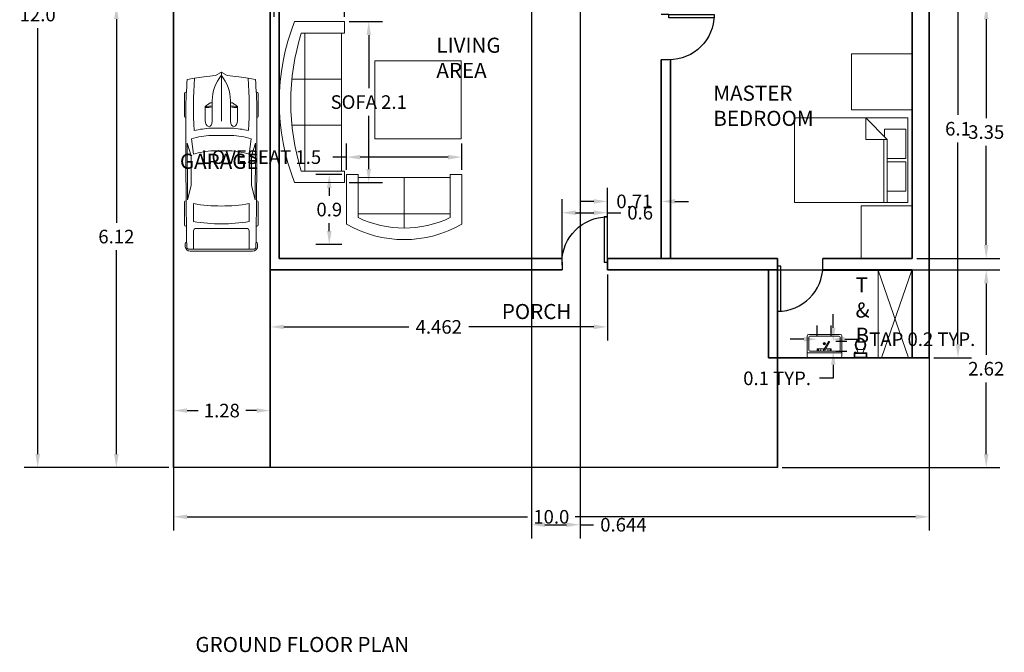
# Model space of a CAD drawing. Units: metres. Extents: x 4.8 to 18.3, y 28.2 to 89.8.
# Tile 1 of 4: x 4.8 to 17.8, y 28.2 to 36.6. Entities that reach past the tile are written whole.
import ezdxf

# ---------------------------------------------------------------- set-up
doc = ezdxf.new("R2010")
doc.units = ezdxf.units.M
doc.header["$MEASUREMENT"] = 0
doc.layers.get('Defpoints').update_dxf_attribs({"color": 3})
for name, color, linetype, lineweight in [('A-ANNO-DIMS', 2, 'Continuous', 18), ('A-ANNO-TEXT', 7, 'Continuous', 25), ('A-AREA-IDEN', 7, 'Continuous', 25), ('A-DOOR', 3, 'Continuous', 25), ('A-EQPM-VEHC', 9, 'Continuous', 13), ('A-FLOR', 8, 'Continuous', 25), ('A-FLOR-FIXT', 9, 'Continuous', 18), ('A-FURN', 8, 'Continuous', 18), ('A-WALL', 7, 'Continuous', 35)]:
    doc.layers.add(name, color=color, linetype=linetype, lineweight=lineweight)
doc.styles.get("Standard").update_dxf_attribs({"font": 'arial.ttf'})
doc.dimstyles.get("Standard").update_dxf_attribs({"dimtxt": 0.18, "dimasz": 0.18, "dimexe": 0.18, "dimexo": 0.0625, "dimgap": 0.09, "dimtad": 0, "dimtih": 1, "dimtoh": 1, "dimdec": 1, "dimzin": 0, "dimdsep": 46, "dimtxsty": 'Standard', "dimcen": 0.09, "dimadec": 0, "dimazin": 0, "dimtfac": 1, "dimtdec": 1, "dimtofl": 0, "dimtmove": 0, "dimatfit": 3, "dimfxl": 1, "dimtolj": 1, "dimtzin": 0, "dimarcsym": 0})

# ---------------------------------------------------------------- blocks, each defined once
blk = doc.blocks.new('Sofa - Roundback 7 ft.')
for p, q in [((-12.00002, -32.4421), (-12.00003, -6.5971)), ((11.99997, -32.4421), (11.99998, -6.5971)), ((-36.000027, -34), (-36.000027, -11.4696)), ((-35.999844, -13.3819), (35.9998, -13.3819)), ((35.99998, -34), (35.99998, -11.4696)), ((-36.000027, -32.4421), (35.99998, -32.4421))]:
    blk.add_line(p, q)
for points in [[(-36.000027, -34), (-42.000027, -34), (-42.000027, -8)], [(41.99998, -8), (41.99998, -34), (35.99998, -34)]]:
    blk.add_lwpolyline(points)
for centre, radius, start, end in [((0, -114.25), 114.25, 68.43141, 111.5686), ((-0.00001, -127.1968), 121.1968, 72.72033, 107.2797)]:
    blk.add_arc(centre, radius, start, end)
blk = doc.blocks.new('Sofa - Roundback Loveseat 5 ft.')
for p, q in [((0, -32.44198), (0, -5.99998)), ((-24, -33.99998), (-24, -11.46958)), ((-23.9998, -13.38178), (23.99986, -13.38178)), ((24.00004, -33.99998), (24.00004, -11.46958)), ((-24, -32.44198), (24.00004, -32.44198))]:
    blk.add_line(p, q)
for points in [[(-24, -33.99998), (-30, -33.99998), (-30, -7.99998)], [(30.00004, -7.99998), (30.00004, -33.99998), (24.00004, -33.99998)]]:
    blk.add_lwpolyline(points)
for centre, radius, start, end in [((0, -60.24998), 60.24998, 60.13715, 119.8628), ((0, -61.38438), 55.38444, 64.32083, 115.6792)]:
    blk.add_arc(centre, radius, start, end)
blk = doc.blocks.new('*U14')
for p, q in [((0, 0), (0, 100)), ((600, 0), (600, 100))]:
    blk.add_line(p, q)
blk.add_lwpolyline([(0, 0), (0, -600), (43.75, -600), (43.75, 0)], close=True)
blk.add_arc((0, 0), 600, 270, 0)
blk = doc.blocks.new('Bed - Queen')
for p, q in [((0, -80.00003), (0, 0)), ((0, 0), (59.99999, 0)), ((59.99999, 0), (59.99999, -80.00003)), ((7.99999, -1.2), (28.79998, -1.2)), ((7.99999, -14.4), (7.99999, -1.2)), ((28.79998, -1.2), (28.79998, -14.4)), ((31.19999, -1.2), (51.99999, -1.2)), ((31.19999, -14.4), (31.19999, -1.2)), ((51.99999, -1.2), (51.99999, -16.4)), ((0, -14.4), (44.8, -14.4)), ((44.8, -16.8), (0, -16.8)), ((59.99999, -29.6), (44.8, -14.4)), ((44.8, -14.4), (44.8, -29.6)), ((51.99999, -16.4), (46.79936, -16.4)), ((44.8, -29.6), (59.99999, -29.6)), ((59.99999, -80.00003), (0, -80.00003))]:
    blk.add_line(p, q)
blk = doc.blocks.new('Toilet - top')
for p, q in [((-10, -8.5), (-8, -8.5)), ((-10, -9.5), (-10, -8.5)), ((-7, -9.5), (-10, -9.5)), ((-8, -8.5), (-8, -8)), ((-7, -8), (-7, -9.5)), ((-4, -8), (-6, -14)), ((4, -14), (-4, -14)), ((4, -8), (6, -14)), ((9.5, -6), (9.5, -2))]:
    blk.add_line(p, q)
blk.add_lwpolyline([(10.5, -8), (10.5, 0), (-10.5, 0), (-10.5, -8)], close=True)
for points in [[(-9.5, -2), (-9.5, -6)], [(8.5, -1), (-8.5, -1)], [(-8.5, -7), (8.5, -7)]]:
    blk.add_lwpolyline(points)
for centre, radius, start, end in [((-8.6, -1.9), 0.884, 81.8699, 188.1301), ((-8.6, -6.1), 0.884, 171.8699, 278.1301), ((3.5, -21.6), 12.2, 141.4691, 247.9714), ((4.2, -21.8), 11.3, 136.3677, 238.9468), ((-3.5, -21.6), 12.2, 292.0284, 38.5307), ((-4.2, -21.8), 11.3, 301.053, 43.6321), ((8.6, -1.9), 0.884, 351.8699, 98.1301), ((8.6, -6.1), 0.884, 261.8699, 8.1301), ((0, -27.9), 4, 245.7318, 294.2682), ((0, -29), 4, 254.8605, 285.1395)]:
    blk.add_arc(centre, radius, start, end)
blk = doc.blocks.new('Sink-single - 30 in top')
blk.add_line((-15, -3.999996), (15, -3.999996))
for points in [[(-13.5, 0), (13.5, 0)], [(-15, -18.499996), (-15, -1.5)], [(-13.5, -17.499996), (-13.5, -6.499996)], [(-12.5, -5.499996), (12.5, -5.499996)], [(13.5, -6.499996), (13.5, -17.499996)], [(15, -1.5), (15, -18.499996)], [(13.5, -19.999996), (-13.5, -19.999996)], [(12.5, -18.499996), (-12.5, -18.499996)]]:
    blk.add_lwpolyline(points)
for radius in [1, 0.5]:
    blk.add_circle((0, -11.999996), radius)
for centre, radius, start, end in [((-13.5, -1.5), 1.5, 90, 180), ((-12.5, -6.499996), 1, 90, 180), ((12.5, -6.499996), 1, 0, 90), ((13.5, -1.5), 1.5, 0, 90), ((-13.5, -18.499996), 1.5, 180, 270), ((-12.5, -17.499996), 1, 180, 270), ((12.5, -17.499996), 1, 270, 0), ((13.5, -18.499996), 1.5, 270, 0)]:
    blk.add_arc(centre, radius, start, end)
blk = doc.blocks.new('Faucet - kit sink top')
for p, q in [((-5.5, -0.75), (-5.5, -1.25)), ((-4.94278, -0.75), (-5.5, -0.75)), ((-5.5, -1.25), (-4.94278, -1.25)), ((-0.14775, -1.7441), (3.56698, -8.1782)), ((4.43301, -7.6782), (0.71828, -1.2441)), ((4.94278, -0.75), (5.5, -0.75)), ((5.5, -1.25), (4.94278, -1.25)), ((5.5, -0.75), (5.5, -1.25))]:
    blk.add_line(p, q)
blk.add_lwpolyline([(-0.00587, -2), (-6, -2), (-6, 0), (6, 0), (6, -2), (1.15195, -2)])
for centre, radius in [((-4, -1), 1), ((4, -1), 1), ((0, -1), 0.75)]:
    blk.add_circle(centre, radius)
blk.add_arc((4, -7.9282), 0.5, 210, 30)
blk = doc.blocks.new('*U15')
for p, q in [((-600, 0), (-600, 100)), ((0, 0), (0, 100))]:
    blk.add_line(p, q)
blk.add_lwpolyline([(0, 0), (0, -600), (-43.75, -600), (-43.75, 0)], close=True)
blk.add_arc((0, 0), 600, 180, 270)
blk = doc.blocks.new('*U17')
for p, q in [((536, 950), (536, 936)), ((1182, 988), (568, 988)), ((1214, 950), (1214, 950)), ((1779, 801), (2195, 746)), ((2235, 810), (1899, 912)), ((3412, 904), (3030, 807)), ((3440, 942), (3440, 950)), ((3472, 988), (4087, 988)), ((4119, 950), (4119, 934)), ((4736, -851), (4736, 851)), ((4785, -832), (4785, 832)), ((3516, 746), (3994, 746)), ((4179, 670), (4179, -670)), ((4736, 746), (4242, 746)), ((816, 241), (816, 283)), ((820, 295), (918, 436)), ((918, 436), (1294, 436)), ((1496, -274), (1496, 274)), ((1690, -267), (1690, 267)), ((4736, -267), (4736, 267)), ((83, 156), (3, 10)), ((756, 241), (1313, 241)), ((2102, 216), (2102, -216)), ((0, 0), (1313, 0)), ((3, -10), (83, -156)), ((756, -241), (1313, -241)), ((816, -241), (816, -283)), ((820, -295), (918, -436)), ((918, -436), (1294, -436)), ((2195, -746), (1779, -801)), ((3994, -746), (3516, -746)), ((4242, -746), (4736, -746)), ((536, -950), (536, -936)), ((1182, -988), (568, -988)), ((1214, -950), (1214, -950)), ((2235, -810), (1899, -912)), ((3412, -904), (3030, -807)), ((3440, -942), (3440, -950)), ((3472, -988), (4087, -988)), ((4119, -950), (4119, -934))]:
    blk.add_line(p, q)
for centre, major_axis, ratio, start_param, end_param in [((6757, -699), (0, 7958), 0.842304, 1.367076, 1.39176), ((1046, -12468), (0, 13417), 0.842304, 0.00281, 0.075598), ((568, 950), (0, -37.6), 0.842304, 3.141593, 4.712389), ((1638, -268113), (0, 269063), 0.842304, -0.013397, 0.002797), ((1182, 950), (0, 37.6), 0.842304, -1.570796, 0), ((3436, 137), (0, 2077), 0.842304, 1.245306, 1.50788), ((1638, -268113), (0, -269025), 0.842304, 3.133765, 3.140441), ((2433, -93125), (0, -93935), 0.842304, 3.134049, 3.144098), ((3472, 950), (0, -37.6), 0.842304, 3.141593, 4.712389), ((4087, 950), (0, 37.6), 0.842304, -1.570796, 0), ((4588, 910), (0, 56.4), 0.842304, -0.013017, 1.249894), ((1638, -268131), (0, 269121), 0.842304, -0.013397, -0.013017), ((4673, 851), (0, -75.2), 0.842304, 1.570796, 3.128196), ((4673, 832), (0, -133), 0.842304, 1.570796, 3.128196), ((6583, -699), (0, -7755), 0.842304, 4.528606, 4.561838), ((952, -15087), (0, -15833), 0.842304, 3.096046, 3.200911), ((3414, 137), (0, -2280), 0.842304, 4.449482, 4.652344), ((3800, 71), (0, -2021), 0.842304, 4.372215, 4.640744), ((434, 0), (0, 3734), 0.842304, 4.511394, 4.913384), ((912, 0), (0, 3734), 0.842304, 4.511394, 4.913384), ((4242, 670), (0, 75.2), 0.842304, 0, 1.570796), ((-5194, 1331), (0, -6374), 0.842304, 1.385369, 1.434372), ((832, 283), (0, 18.8), 0.842304, 0.879714, 1.570796), ((331, 432), (0, 696), 0.842304, 4.435146, 4.718221), ((361, 432), (0, 696), 0.842304, 4.435146, 4.718221), ((1290, 339), (161, -9), 0.603834, -1.395552, 1.581315), ((16, 0), (0, -18.8), 0.842304, 4.131459, 5.293319), ((756, -1185), (0, 1427), 0.842304, 0, 0.590319), ((-5194, -1331), (0, 6374), 0.842304, -1.434372, -1.385369), ((756, 1185), (0, 1427), 0.842304, 2.551274, 3.141593), ((331, -432), (0, -696), 0.842304, 1.564964, 1.848039), ((361, -432), (0, -696), 0.842304, 1.564964, 1.848039), ((3800, -71), (0, -2021), 0.842304, -1.499151, -1.230623), ((6583, 699), (0, 7755), 0.842304, 1.721348, 1.754579), ((832, -283), (0, -18.8), 0.842304, 4.712389, 5.403472), ((3414, -137), (0, -2280), 0.842304, -1.510751, -1.307889), ((3436, -137), (0, -2077), 0.842304, -1.50788, -1.245306), ((6757, 699), (0, 7958), 0.842304, 1.749832, 1.774517), ((952, 15087), (0, -15833), 0.842304, -0.059319, 0.045547), ((4242, -670), (0, -75.2), 0.842304, 4.712389, 6.283185), ((1046, 12468), (0, -13417), 0.842304, -0.075598, -0.00281), ((568, -950), (0, 37.6), 0.842304, 1.570796, 3.141593), ((1638, 268113), (0, 269063), 0.842304, 3.138796, 3.15499), ((1182, -950), (0, -37.6), 0.842304, 0, 1.570796), ((1638, 268113), (0, -269025), 0.842304, 0.001152, 0.007828), ((2433, 93125), (0, -93935), 0.842304, -0.002505, 0.007544), ((3472, -950), (0, -37.6), 0.842304, -1.570796, 0), ((4087, -950), (0, 37.6), 0.842304, 3.141593, 4.712389), ((4588, -910), (0, -56.4), 0.842304, -1.249894, 0.013017), ((1638, 268131), (0, 269121), 0.842304, 3.15461, 3.15499), ((4673, -851), (0, 75.2), 0.842304, 3.15499, 4.712389), ((4673, -832), (0, -133), 0.842304, 0.013397, 1.570796)]:
    blk.add_ellipse(centre, major_axis=major_axis, ratio=ratio, start_param=start_param, end_param=end_param)
at = {"extrusion": (0, 0, -1)}
blk.add_ellipse((1290, -339), major_axis=(161, 9), ratio=0.603834, start_param=-1.395552, end_param=1.581315, dxfattribs=at)
blk = doc.blocks.new('*D18')
at = {"layer": 'A-ANNO-DIMS', "color": 0, "lineweight": -2, "transparency": 16777216}
for p, q in [((6.731, 42.663), (4.816, 42.663)), ((4.996, 42.483), (4.996, 36.845)), ((4.996, 30.843), (4.996, 36.481)), ((6.731, 30.663), (4.816, 30.663))]:
    blk.add_line(p, q, dxfattribs=at)
at = {"layer": 'A-ANNO-DIMS', "color": 0, "transparency": 16777216}
for points in [[(4.966, 42.483), (5.026, 42.483), (4.996, 42.663)], [(4.966, 30.843), (5.026, 30.843), (4.996, 30.663)]]:
    blk.add_solid(points, dxfattribs=at)
at = {"layer": 'Defpoints', "color": 0, "transparency": 16777216}
for p in [(6.793, 42.663), (4.996, 30.663), (6.793, 30.663)]:
    blk.add_point(p, dxfattribs=at)
at = {"layer": 'A-ANNO-DIMS', "color": 0, "transparency": 16777216, "insert": (4.996, 36.663), "char_height": 0.18, "attachment_point": 5}
blk.add_mtext('\\A1;12.0', dxfattribs=at)
blk = doc.blocks.new('*D19')
at = {"layer": 'A-ANNO-DIMS', "color": 0, "lineweight": -2, "transparency": 16777216}
for p, q in [((6.793, 33.404), (6.793, 29.832)), ((16.793, 33.369), (16.793, 29.832)), ((6.973, 30.012), (11.478, 30.012)), ((16.613, 30.012), (12.108, 30.012))]:
    blk.add_line(p, q, dxfattribs=at)
at = {"layer": 'A-ANNO-DIMS', "color": 0, "transparency": 16777216}
for points in [[(6.973, 30.042), (6.973, 29.982), (6.793, 30.012)], [(16.613, 30.042), (16.613, 29.982), (16.793, 30.012)]]:
    blk.add_solid(points, dxfattribs=at)
at = {"layer": 'Defpoints', "color": 0, "transparency": 16777216}
for p in [(6.793, 33.467), (16.793, 33.432), (6.793, 30.012)]:
    blk.add_point(p, dxfattribs=at)
at = {"layer": 'A-ANNO-DIMS', "color": 0, "transparency": 16777216, "insert": (11.793, 30.012), "char_height": 0.18, "attachment_point": 5}
blk.add_mtext('\\A1;10.0', dxfattribs=at)
blk = doc.blocks.new('*D20')
at = {"layer": 'A-ANNO-DIMS', "color": 0, "lineweight": -2, "transparency": 16777216}
for p, q in [((16.856, 38.183), (17.355, 38.183)), ((17.175, 38.003), (17.175, 35.333)), ((17.175, 32.299), (17.175, 34.969)), ((16.856, 32.119), (17.355, 32.119))]:
    blk.add_line(p, q, dxfattribs=at)
at = {"layer": 'A-ANNO-DIMS', "color": 0, "transparency": 16777216}
for points in [[(17.145, 38.003), (17.205, 38.003), (17.175, 38.183)], [(17.145, 32.299), (17.205, 32.299), (17.175, 32.119)]]:
    blk.add_solid(points, dxfattribs=at)
at = {"layer": 'Defpoints', "color": 0, "transparency": 16777216}
for p in [(16.793, 38.183), (16.793, 32.119), (17.175, 32.119)]:
    blk.add_point(p, dxfattribs=at)
at = {"layer": 'A-ANNO-DIMS', "color": 0, "transparency": 16777216, "insert": (17.175, 35.151), "char_height": 0.18, "attachment_point": 5}
blk.add_mtext('\\A1;6.1', dxfattribs=at)
blk = doc.blocks.new('*D34')
at = {"layer": 'A-ANNO-DIMS', "color": 0, "lineweight": -2, "transparency": 16777216}
for p, q in [((15.313, 32.399), (15.313, 32.544)), ((15.497, 32.399), (15.497, 32.544)), ((15.133, 32.364), (14.953, 32.364)), ((15.677, 32.364), (15.857, 32.364))]:
    blk.add_line(p, q, dxfattribs=at)
at = {"layer": 'A-ANNO-DIMS', "color": 0, "transparency": 16777216}
for points in [[(15.133, 32.394), (15.133, 32.334), (15.313, 32.364)], [(15.677, 32.394), (15.677, 32.334), (15.497, 32.364)]]:
    blk.add_solid(points, dxfattribs=at)
at = {"layer": 'Defpoints', "color": 0, "transparency": 16777216}
for p in [(15.313, 32.336), (15.497, 32.364), (15.497, 32.336)]:
    blk.add_point(p, dxfattribs=at)
at = {"layer": 'A-ANNO-DIMS', "color": 0, "transparency": 16777216, "insert": (16.702, 32.364), "char_height": 0.18, "attachment_point": 5}
blk.add_mtext('\\A1;TAP 0.2 TYP.', dxfattribs=at)
blk = doc.blocks.new('*D35')
at = {"layer": 'A-ANNO-DIMS', "color": 0, "lineweight": -2, "transparency": 16777216}
for p, q in [((15.524, 32.516), (15.524, 32.696)), ((15.559, 32.336), (15.704, 32.336)), ((15.559, 32.206), (15.704, 32.206)), ((15.524, 32.026), (15.524, 31.846)), ((15.524, 31.846), (15.344, 31.846))]:
    blk.add_line(p, q, dxfattribs=at)
at = {"layer": 'A-ANNO-DIMS', "color": 0, "transparency": 16777216}
for points in [[(15.494, 32.516), (15.554, 32.516), (15.524, 32.336)], [(15.494, 32.026), (15.554, 32.026), (15.524, 32.206)]]:
    blk.add_solid(points, dxfattribs=at)
at = {"layer": 'Defpoints', "color": 0, "transparency": 16777216}
for p in [(15.497, 32.336), (15.497, 32.206), (15.524, 32.206)]:
    blk.add_point(p, dxfattribs=at)
at = {"layer": 'A-ANNO-DIMS', "color": 0, "transparency": 16777216, "insert": (14.781, 31.846), "char_height": 0.18, "attachment_point": 5}
blk.add_mtext('\\A1;0.1 TYP.', dxfattribs=at)
blk = doc.blocks.new('*D40')
at = {"layer": 'A-ANNO-DIMS', "color": 0, "lineweight": -2, "transparency": 16777216}
for p, q in [((9.119, 36.571), (9.557, 36.571)), ((9.377, 36.391), (9.377, 35.687)), ((9.377, 34.617), (9.377, 35.321)), ((9.119, 34.437), (9.557, 34.437))]:
    blk.add_line(p, q, dxfattribs=at)
at = {"layer": 'A-ANNO-DIMS', "color": 0, "transparency": 16777216}
for points in [[(9.347, 36.391), (9.407, 36.391), (9.377, 36.571)], [(9.347, 34.617), (9.407, 34.617), (9.377, 34.437)]]:
    blk.add_solid(points, dxfattribs=at)
at = {"layer": 'Defpoints', "color": 0, "transparency": 16777216}
for p in [(9.057, 36.571), (9.377, 36.571), (9.057, 34.437)]:
    blk.add_point(p, dxfattribs=at)
at = {"layer": 'A-ANNO-DIMS', "color": 0, "transparency": 16777216, "insert": (9.377, 35.504), "char_height": 0.18, "attachment_point": 5}
blk.add_mtext('\\A1;SOFA 2.1', dxfattribs=at)
blk = doc.blocks.new('*D41')
at = {"layer": 'A-ANNO-DIMS', "color": 0, "lineweight": -2, "transparency": 16777216}
for p, q in [((8.125, 36.633), (8.125, 37.071)), ((9.057, 36.633), (9.057, 37.071)), ((8.125, 36.891), (7.945, 36.891)), ((8.877, 36.891), (8.305, 36.891))]:
    blk.add_line(p, q, dxfattribs=at)
at = {"layer": 'A-ANNO-DIMS', "color": 0, "transparency": 16777216}
for points in [[(8.305, 36.921), (8.305, 36.861), (8.125, 36.891)], [(8.877, 36.921), (8.877, 36.861), (9.057, 36.891)]]:
    blk.add_solid(points, dxfattribs=at)
at = {"layer": 'Defpoints', "color": 0, "transparency": 16777216}
for p in [(8.125, 36.891), (8.125, 36.571), (9.057, 36.571)]:
    blk.add_point(p, dxfattribs=at)
at = {"layer": 'A-ANNO-DIMS', "color": 0, "transparency": 16777216, "insert": (7.691, 36.891), "char_height": 0.18, "attachment_point": 5}
blk.add_mtext('\\A1;0.9', dxfattribs=at)
blk = doc.blocks.new('*D42')
at = {"layer": 'A-ANNO-DIMS', "color": 0, "lineweight": -2, "transparency": 16777216}
for p, q in [((9.084, 34.609), (9.084, 34.955)), ((10.608, 34.609), (10.608, 34.955)), ((9.084, 34.775), (8.904, 34.775)), ((10.428, 34.775), (9.264, 34.775))]:
    blk.add_line(p, q, dxfattribs=at)
at = {"layer": 'A-ANNO-DIMS', "color": 0, "transparency": 16777216}
for points in [[(9.264, 34.805), (9.264, 34.745), (9.084, 34.775)], [(10.428, 34.805), (10.428, 34.745), (10.608, 34.775)]]:
    blk.add_solid(points, dxfattribs=at)
at = {"layer": 'Defpoints', "color": 0, "transparency": 16777216}
for p in [(9.084, 34.775), (9.084, 34.547), (10.608, 34.547)]:
    blk.add_point(p, dxfattribs=at)
at = {"layer": 'A-ANNO-DIMS', "color": 0, "transparency": 16777216, "insert": (7.955, 34.775), "char_height": 0.18, "attachment_point": 5}
blk.add_mtext('\\A1;LOVESEAT 1.5', dxfattribs=at)
blk = doc.blocks.new('*D43')
at = {"layer": 'A-ANNO-DIMS', "color": 0, "lineweight": -2, "transparency": 16777216}
for p, q in [((9.021, 34.547), (8.675, 34.547)), ((8.855, 34.367), (8.855, 34.263)), ((8.855, 33.796), (8.855, 33.899)), ((9.021, 33.616), (8.675, 33.616))]:
    blk.add_line(p, q, dxfattribs=at)
at = {"layer": 'A-ANNO-DIMS', "color": 0, "transparency": 16777216}
for points in [[(8.825, 34.367), (8.885, 34.367), (8.855, 34.547)], [(8.825, 33.796), (8.885, 33.796), (8.855, 33.616)]]:
    blk.add_solid(points, dxfattribs=at)
at = {"layer": 'Defpoints', "color": 0, "transparency": 16777216}
for p in [(9.084, 34.547), (8.855, 33.616), (9.084, 33.616)]:
    blk.add_point(p, dxfattribs=at)
at = {"layer": 'A-ANNO-DIMS', "color": 0, "transparency": 16777216, "insert": (8.855, 34.081), "char_height": 0.18, "attachment_point": 5}
blk.add_mtext('\\A1;0.9', dxfattribs=at)
blk = doc.blocks.new('*D46')
at = {"layer": 'A-ANNO-DIMS', "color": 0, "lineweight": -2, "transparency": 16777216}
for p, q in [((6.793, 30.726), (6.793, 31.599)), ((8.073, 30.726), (8.073, 31.599)), ((6.973, 31.419), (7.118, 31.419)), ((7.893, 31.419), (7.749, 31.419))]:
    blk.add_line(p, q, dxfattribs=at)
at = {"layer": 'A-ANNO-DIMS', "color": 0, "transparency": 16777216}
for points in [[(6.973, 31.449), (6.973, 31.389), (6.793, 31.419)], [(7.893, 31.449), (7.893, 31.389), (8.073, 31.419)]]:
    blk.add_solid(points, dxfattribs=at)
at = {"layer": 'Defpoints', "color": 0, "transparency": 16777216}
for p in [(8.073, 31.419), (6.793, 30.663), (8.073, 30.663)]:
    blk.add_point(p, dxfattribs=at)
at = {"layer": 'A-ANNO-DIMS', "color": 0, "transparency": 16777216, "insert": (7.433, 31.419), "char_height": 0.18, "attachment_point": 5}
blk.add_mtext('\\A1;1.28', dxfattribs=at)
blk = doc.blocks.new('*D47')
at = {"layer": 'A-ANNO-DIMS', "color": 0, "lineweight": -2, "transparency": 16777216}
for p, q in [((6.731, 36.783), (5.857, 36.783)), ((6.037, 36.603), (6.037, 33.905)), ((6.037, 30.843), (6.037, 33.541)), ((6.731, 30.663), (5.857, 30.663))]:
    blk.add_line(p, q, dxfattribs=at)
at = {"layer": 'A-ANNO-DIMS', "color": 0, "transparency": 16777216}
for points in [[(6.007, 36.603), (6.067, 36.603), (6.037, 36.783)], [(6.007, 30.843), (6.067, 30.843), (6.037, 30.663)]]:
    blk.add_solid(points, dxfattribs=at)
at = {"layer": 'Defpoints', "color": 0, "transparency": 16777216}
for p in [(6.037, 36.783), (6.793, 36.783), (6.793, 30.663)]:
    blk.add_point(p, dxfattribs=at)
at = {"layer": 'A-ANNO-DIMS', "color": 0, "transparency": 16777216, "insert": (6.037, 33.723), "char_height": 0.18, "attachment_point": 5}
blk.add_mtext('\\A1;6.12', dxfattribs=at)
blk = doc.blocks.new('*D48')
at = {"layer": 'A-ANNO-DIMS', "color": 0, "lineweight": -2, "transparency": 16777216}
for p, q in [((14.73, 33.283), (17.729, 33.283)), ((17.549, 33.103), (17.549, 32.155)), ((17.549, 30.843), (17.549, 31.791)), ((14.85, 30.663), (17.729, 30.663))]:
    blk.add_line(p, q, dxfattribs=at)
at = {"layer": 'A-ANNO-DIMS', "color": 0, "transparency": 16777216}
for points in [[(17.519, 33.103), (17.579, 33.103), (17.549, 33.283)], [(17.519, 30.843), (17.579, 30.843), (17.549, 30.663)]]:
    blk.add_solid(points, dxfattribs=at)
at = {"layer": 'Defpoints', "color": 0, "transparency": 16777216}
for p in [(14.667, 33.283), (17.549, 33.283), (14.787, 30.663)]:
    blk.add_point(p, dxfattribs=at)
at = {"layer": 'A-ANNO-DIMS', "color": 0, "transparency": 16777216, "insert": (17.549, 31.973), "char_height": 0.18, "attachment_point": 5}
blk.add_mtext('\\A1;2.62', dxfattribs=at)
blk = doc.blocks.new('*D49')
at = {"layer": 'A-ANNO-DIMS', "color": 0, "lineweight": -2, "transparency": 16777216}
for p, q in [((8.073, 33.221), (8.073, 32.347)), ((12.535, 33.221), (12.535, 32.347)), ((8.253, 32.527), (9.908, 32.527)), ((12.355, 32.527), (10.701, 32.527))]:
    blk.add_line(p, q, dxfattribs=at)
at = {"layer": 'A-ANNO-DIMS', "color": 0, "transparency": 16777216}
for points in [[(8.253, 32.557), (8.253, 32.497), (8.073, 32.527)], [(12.355, 32.557), (12.355, 32.497), (12.535, 32.527)]]:
    blk.add_solid(points, dxfattribs=at)
at = {"layer": 'Defpoints', "color": 0, "transparency": 16777216}
for p in [(8.073, 33.283), (12.535, 33.283), (8.073, 32.527)]:
    blk.add_point(p, dxfattribs=at)
at = {"layer": 'A-ANNO-DIMS', "color": 0, "transparency": 16777216, "insert": (10.304, 32.527), "char_height": 0.18, "attachment_point": 5}
blk.add_mtext('\\A1;4.462', dxfattribs=at)
blk = doc.blocks.new('*D50')
at = {"layer": 'A-ANNO-DIMS', "color": 0, "lineweight": -2, "transparency": 16777216}
for p, q in [((16.631, 36.782), (17.729, 36.782)), ((17.549, 36.602), (17.549, 35.289)), ((17.549, 33.612), (17.549, 34.925)), ((16.631, 33.432), (17.729, 33.432))]:
    blk.add_line(p, q, dxfattribs=at)
at = {"layer": 'A-ANNO-DIMS', "color": 0, "transparency": 16777216}
for points in [[(17.519, 36.602), (17.579, 36.602), (17.549, 36.782)], [(17.519, 33.612), (17.579, 33.612), (17.549, 33.432)]]:
    blk.add_solid(points, dxfattribs=at)
at = {"layer": 'Defpoints', "color": 0, "transparency": 16777216}
for p in [(16.568, 36.782), (17.549, 36.782), (16.568, 33.432)]:
    blk.add_point(p, dxfattribs=at)
at = {"layer": 'A-ANNO-DIMS', "color": 0, "transparency": 16777216, "insert": (17.549, 35.107), "char_height": 0.18, "attachment_point": 5}
blk.add_mtext('\\A1;3.35', dxfattribs=at)
blk = doc.blocks.new('*D56')
at = {"layer": 'A-ANNO-DIMS', "color": 0, "lineweight": -2, "transparency": 16777216}
for p, q in [((11.935, 33.346), (11.935, 34.219)), ((12.535, 33.346), (12.535, 34.219)), ((12.115, 34.039), (12.355, 34.039)), ((12.535, 34.039), (12.715, 34.039))]:
    blk.add_line(p, q, dxfattribs=at)
at = {"layer": 'A-ANNO-DIMS', "color": 0, "transparency": 16777216}
for points in [[(12.115, 34.069), (12.115, 34.009), (11.935, 34.039)], [(12.355, 34.069), (12.355, 34.009), (12.535, 34.039)]]:
    blk.add_solid(points, dxfattribs=at)
at = {"layer": 'Defpoints', "color": 0, "transparency": 16777216}
for p in [(12.535, 34.039), (11.935, 33.283), (12.535, 33.283)]:
    blk.add_point(p, dxfattribs=at)
at = {"layer": 'A-ANNO-DIMS', "color": 0, "transparency": 16777216, "insert": (12.969, 34.039), "char_height": 0.18, "attachment_point": 5}
blk.add_mtext('\\A1;0.6', dxfattribs=at)
blk = doc.blocks.new('*D57')
at = {"layer": 'A-ANNO-DIMS', "color": 0, "lineweight": -2, "transparency": 16777216}
for p, q in [((12.535, 33.496), (12.535, 34.369)), ((13.248, 33.496), (13.248, 34.369)), ((12.355, 34.189), (12.175, 34.189)), ((13.428, 34.189), (13.608, 34.189))]:
    blk.add_line(p, q, dxfattribs=at)
at = {"layer": 'A-ANNO-DIMS', "color": 0, "transparency": 16777216}
for points in [[(12.355, 34.219), (12.355, 34.159), (12.535, 34.189)], [(13.428, 34.219), (13.428, 34.159), (13.248, 34.189)]]:
    blk.add_solid(points, dxfattribs=at)
at = {"layer": 'Defpoints', "color": 0, "transparency": 16777216}
for p in [(13.248, 34.189), (12.535, 33.433), (13.248, 33.433)]:
    blk.add_point(p, dxfattribs=at)
at = {"layer": 'A-ANNO-DIMS', "color": 0, "transparency": 16777216, "insert": (12.892, 34.189), "char_height": 0.18, "attachment_point": 5}
blk.add_mtext('\\A1;0.71', dxfattribs=at)
blk = doc.blocks.new('*D60')
at = {"layer": 'A-ANNO-DIMS', "color": 0, "lineweight": -2, "transparency": 16777216}
for p, q in [((12.173, 41.648), (12.173, 29.727)), ((11.529, 41.382), (11.529, 29.727)), ((11.709, 29.907), (11.993, 29.907)), ((12.173, 29.907), (12.353, 29.907))]:
    blk.add_line(p, q, dxfattribs=at)
at = {"layer": 'A-ANNO-DIMS', "color": 0, "transparency": 16777216}
for points in [[(11.709, 29.937), (11.709, 29.877), (11.529, 29.907)], [(11.993, 29.937), (11.993, 29.877), (12.173, 29.907)]]:
    blk.add_solid(points, dxfattribs=at)
at = {"layer": 'Defpoints', "color": 0, "transparency": 16777216}
for p in [(12.173, 41.711), (11.529, 41.445), (12.173, 29.907)]:
    blk.add_point(p, dxfattribs=at)
at = {"layer": 'A-ANNO-DIMS', "color": 0, "transparency": 16777216, "insert": (12.747, 29.907), "char_height": 0.18, "attachment_point": 5}
blk.add_mtext('\\A1;0.644', dxfattribs=at)

msp = doc.modelspace()

# ---------------------------------------------------------------- linework, layer by layer
at = {"layer": 'A-FLOR'}
msp.add_line((14.7874, 30.6633), (6.7935, 30.6633), dxfattribs=at)
at = {"layer": 'A-FLOR-FIXT'}
for p, q in [((16.1198, 33.2794), (16.1198, 32.1194)), ((16.1198, 33.2794), (16.5206, 32.1194)), ((16.1616, 32.1194), (16.5624, 33.2794))]:
    msp.add_line(p, q, dxfattribs=at)
at = {"layer": 'A-FURN'}
for points in [[(16.5685, 35.4013), (15.7653, 35.4013), (15.7653, 36.1418), (16.5685, 36.1418)], [(9.4562, 36.0509), (10.6001, 36.0509), (10.6001, 35.0168), (9.4562, 35.0168)], [(16.5685, 33.4322), (15.894, 33.4322), (15.894, 34.129), (16.5685, 34.129)]]:
    msp.add_lwpolyline(points, close=True, dxfattribs=at)
at = {"layer": 'A-WALL'}
for p, q in [((6.7935, 30.6633), (6.7935, 42.6633)), ((16.5685, 38.1833), (16.5685, 33.4322)), ((16.7935, 38.1833), (16.7935, 32.1194)), ((8.1935, 33.4333), (8.1935, 36.9033)), ((8.0735, 30.6633), (8.0735, 36.7833)), ((13.2485, 36.0633), (13.2485, 33.4333)), ((13.3685, 36.0636), (13.3685, 33.4333)), ((8.1935, 33.4333), (11.9374, 33.4333)), ((12.5353, 33.4333), (12.5353, 33.2833)), ((12.5353, 33.4333), (14.7874, 33.4333)), ((14.7874, 30.6633), (14.7874, 33.4333)), ((15.3874, 33.4333), (16.126, 33.4333)), ((15.3931, 33.4322), (16.5685, 33.4322)), ((8.0735, 33.2833), (11.9353, 33.2833)), ((12.5353, 33.2833), (14.7874, 33.2833)), ((14.6674, 32.1194), (14.6674, 33.2833)), ((15.3849, 33.2794), (16.5624, 33.2794)), ((15.3931, 33.2822), (16.5685, 33.2822)), ((16.5685, 33.2822), (16.5685, 32.1194)), ((14.6674, 32.1194), (16.7935, 32.1194)), ((14.7674, 32.1194), (14.7874, 32.1194))]:
    msp.add_line(p, q, dxfattribs=at)

# ---------------------------------------------------------------- block references
at = {"layer": 'A-DOOR', "xscale": -0.001, "yscale": 0.001, "zscale": 0.001}
for name, p, rotation in [('*U14', (13.3485, 36.6633), 90), ('*U15', (12.5353, 33.3833), 180)]:
    msp.add_blockref(name, p, dxfattribs=dict(at, rotation=rotation))
at = {"layer": 'A-DOOR', "xscale": 0.001, "yscale": 0.001, "zscale": 0.001}
msp.add_blockref('*U14', (14.7874, 33.3333), dxfattribs=at)
at = {"layer": 'A-EQPM-VEHC', "xscale": 0.0004948326892598, "yscale": 0.0004948326892598, "zscale": 0.0004948326892598, "rotation": 270}
msp.add_blockref('*U17', (7.4263, 35.899), dxfattribs=at)
at = {"layer": 'A-FLOR-FIXT', "rotation": 180}
for name, p, xscale, yscale, zscale in [('Sink-single - 30 in top', (15.4078, 32.1213), -0.0153508848932381, 0.0153508848932381, 0.0153508848932381), ('Faucet - kit sink top', (15.4047, 32.2058), -0.0153508848932381, 0.0153508848932381, 0.0153508848932381), ('Toilet - top', (15.8847, 32.118), -0.0079224064411582, 0.0079224064411582, 0.0079224064411582)]:
    msp.add_blockref(name, p, dxfattribs=dict(at, xscale=xscale, yscale=yscale, zscale=zscale))
at = {"layer": 'A-FURN'}
for name, p, xscale, yscale, zscale, rotation in [('Sofa - Roundback 7 ft.', (8.1929, 35.5042), 0.0254, 0.0254, 0.0254, 90), ('Bed - Queen', (16.5092, 34.1726), -0.0187047454928596, 0.0187047454928596, 0.0187047454928596, 270), ('Sofa - Roundback Loveseat 5 ft.', (9.8459, 33.6832), 0.0254, 0.0254, 0.0254, 180)]:
    msp.add_blockref(name, p, dxfattribs=dict(at, xscale=xscale, yscale=yscale, zscale=zscale, rotation=rotation))

# ---------------------------------------------------------------- texts
at = {"layer": 'A-ANNO-TEXT', "insert": (7.0829, 28.4212), "char_height": 0.2, "attachment_point": 1}
msp.add_mtext_dynamic_manual_height_columns('GROUND FLOOR PLAN', width=12.354327, gutter_width=1, heights=[0], dxfattribs=at)
at = {"layer": 'A-AREA-IDEN', "char_height": 0.2, "attachment_point": 1}
for s, width, insert in [('LIVING AREA', 0.829678, (10.2718, 36.3569)), ('MASTER BEDROOM', 0.829678, (13.9368, 35.7222)), ('GARAGE', 0.334444, (6.8774, 34.82)), ('T & B', 0.334444, (15.8194, 33.1835)), ('PORCH', 0.334444, (11.1379, 32.8304))]:
    msp.add_mtext_dynamic_manual_height_columns(s, width=width, gutter_width=1, heights=[0], dxfattribs=dict(at, insert=insert))

# ---------------------------------------------------------------- dimensions: what is measured, and where the dimension line sits
at = {"layer": 'A-ANNO-DIMS'}
for base, p1, p2, angle, override, picture, middle in [((4.9963, 30.6633), (6.7935, 42.6633), (6.7935, 30.6633), 90, {"dimclrd": 0, "dimclre": 0, "dimclrt": 0}, '*D18', (4.9963, 36.6633)), ((17.175, 32.1194), (16.7935, 38.1833), (16.7935, 32.1194), 90, {"dimclrd": 0, "dimclre": 0, "dimclrt": 0}, '*D20', (17.175, 35.1513)), ((8.1252, 36.891), (9.0565, 36.571), (8.1252, 36.571), 180, {"dimdec": 1, "dimlfac": 1, "dimrnd": 0, "dimzin": 0, "dimdsep": 46, "dimlunit": 2}, '*D41', (7.6911, 36.891)), ((6.0375, 36.7833), (6.7935, 30.6633), (6.7935, 36.7833), 90, {"dimdec": 2, "dimlfac": 1, "dimrnd": 0, "dimzin": 0, "dimdsep": 46, "dimlunit": 2}, '*D47', (6.0375, 33.7233)), ((17.5495, 36.7822), (16.5685, 33.4322), (16.5685, 36.7822), 90, {"dimdec": 2, "dimlfac": 1, "dimrnd": 0, "dimzin": 0, "dimdsep": 46, "dimlunit": 2}, '*D50', (17.5495, 35.1072)), ((8.8553, 33.6155), (9.0839, 34.5468), (9.0839, 33.6155), 270, {"dimdec": 1, "dimlfac": 1, "dimrnd": 0, "dimzin": 0, "dimdsep": 46, "dimlunit": 2}, '*D43', (8.8553, 34.0812)), ((8.0735, 32.5273), (12.5353, 33.2833), (8.0735, 33.2833), 180, {"dimdec": 3, "dimlfac": 1, "dimrnd": 0, "dimzin": 0, "dimdsep": 46, "dimlunit": 2}, '*D49', (10.3044, 32.5273)), ((17.5495, 33.2833), (14.7874, 30.6633), (14.6674, 33.2833), 90, {"dimdec": 2, "dimlfac": 1, "dimrnd": 0, "dimzin": 0, "dimdsep": 46, "dimlunit": 2}, '*D48', (17.5495, 31.9733))]:
    dim = msp.add_linear_dim(base=base, p1=p1, p2=p2, angle=angle, dimstyle='Standard', override=override, dxfattribs=at)
    dim.commit()
    dim.dimension.update_dxf_attribs({"geometry": picture, "text_midpoint": middle})
for base, p1, p2, override, picture, middle in [((12.1735, 29.9073), (11.5294, 41.4446), (12.1735, 41.711), {"dimdec": 3, "dimlfac": 1, "dimrnd": 0, "dimzin": 0, "dimdsep": 46, "dimlunit": 2}, '*D60', (12.7468, 29.9073)), ((13.2485, 34.1893), (12.5353, 33.4333), (13.2485, 33.4333), {"dimdec": 2, "dimlfac": 1, "dimrnd": 0, "dimzin": 0, "dimdsep": 46, "dimlunit": 2}, '*D57', (12.8919, 34.1893)), ((12.5353, 34.0393), (11.9353, 33.2833), (12.5353, 33.2833), {"dimdec": 1, "dimlfac": 1, "dimrnd": 0, "dimzin": 0, "dimdsep": 46, "dimlunit": 2}, '*D56', (12.9691, 34.0393)), ((6.7935, 30.0125), (16.7935, 33.4317), (6.7935, 33.4666), {"dimclrd": 0, "dimclre": 0, "dimclrt": 0}, '*D19', (11.7935, 30.0125)), ((8.0735, 31.4193), (6.7935, 30.6633), (8.0735, 30.6633), {"dimdec": 2, "dimlfac": 1, "dimrnd": 0, "dimzin": 0, "dimdsep": 46, "dimlunit": 2}, '*D46', (7.4335, 31.4193))]:
    dim = msp.add_linear_dim(base=base, p1=p1, p2=p2, dimstyle='Standard', override=override, dxfattribs=at)
    dim.commit()
    dim.dimension.update_dxf_attribs({"geometry": picture, "text_midpoint": middle})
for base, p1, p2, angle, text, picture, middle in [((9.3766, 36.571), (9.0565, 34.4374), (9.0565, 36.571), 90, 'SOFA <>', '*D40', (9.3766, 35.5042)), ((9.0839, 34.7754), (10.6079, 34.5468), (9.0839, 34.5468), 180, 'LOVESEAT <>', '*D42', (7.9546, 34.7754)), ((15.5245, 32.2058), (15.4968, 32.3362), (15.4968, 32.2058), 270, '<> TYP.', '*D35', (14.7814, 31.8458))]:
    dim = msp.add_linear_dim(base=base, p1=p1, p2=p2, angle=angle, text=text, dimstyle='Standard', override={"dimdec": 1, "dimlfac": 1, "dimrnd": 0, "dimzin": 0, "dimdsep": 46, "dimlunit": 2}, dxfattribs=at)
    dim.commit()
    dim.dimension.update_dxf_attribs({"geometry": picture, "text_midpoint": middle})
dim = msp.add_linear_dim(base=(15.4968, 32.3639), p1=(15.3126, 32.3362), p2=(15.4968, 32.3362), text='TAP <> TYP.', dimstyle='Standard', override={"dimdec": 1, "dimlfac": 1, "dimrnd": 0, "dimzin": 0, "dimdsep": 46, "dimlunit": 2}, dxfattribs=at)
dim.commit()
dim.dimension.update_dxf_attribs({"geometry": '*D34', "text_midpoint": (16.7016, 32.3639)})

doc.saveas('drawing.dxf')
